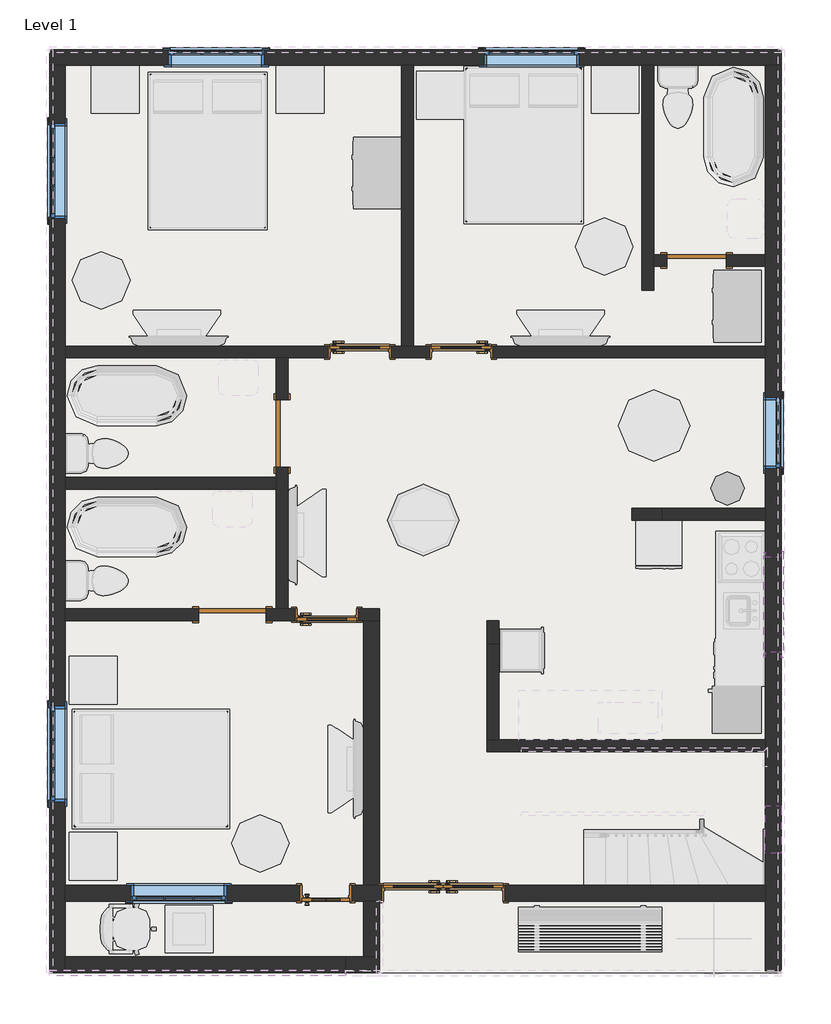
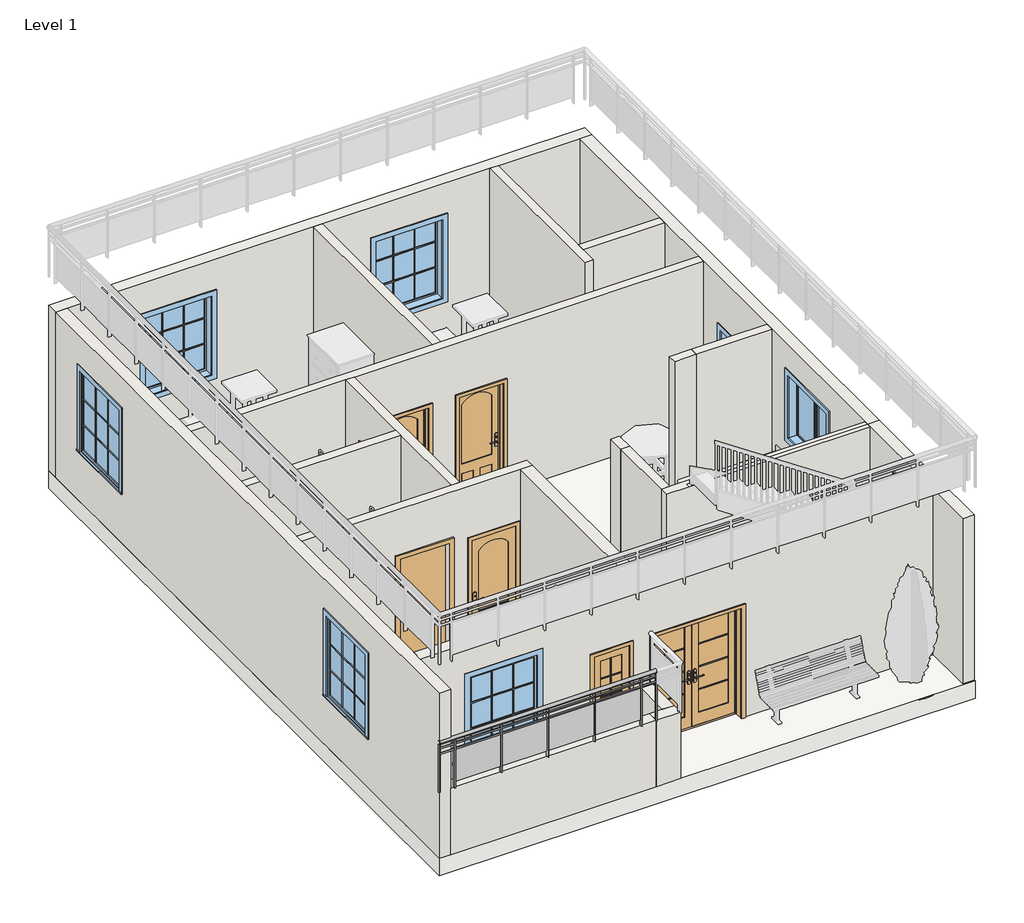
# One storey, part 1 of 4: 20 walls, 8 doors, 8 windows, 1 railing, 1 slab.
"""IFC4 building model written with IfcOpenShell, lengths in millimetres."""

from ifc_helpers import new_model, si_unit, point, frame, origin, origin_with_axes, place, context, project, spatial, polyline, ellipse_curve, trimmed, outline, extrude, faceted_brep, transform, mapped, element, save
from ifc_brep_helpers import plane_surface, extruded_surface, advanced_brep
from components import door_14b9be53, door_4b146b56, door_b03bd389, door_4bd6b2e0, door_255cab33, door_99d96fc5, door_b6e9fca3, window_29c06734, window_99fc0ff6, window_0862ab64, window_6846e476

model = new_model("IFC4")

# Units and contexts
model_context = context("Model", 3, world=origin())
ifc_project = project(units=[si_unit("LENGTHUNIT", "METRE", prefix="MILLI")], contexts=[model_context])

# Site, building, storey
site = spatial("IfcSite", under=ifc_project)
building = spatial("IfcBuilding", under=site)
storey = spatial("IfcBuildingStorey", under=building, Name="Level 1", Elevation=0.0)

# Doors
placement = place(None, origin())
door_shape = door_14b9be53(model_context)
element("IfcDoor", 1, ObjectType="30\" x 80\"", at=placement, inside=storey, context=model_context, shape_type="MappedRepresentation", body=[
    mapped(door_shape, transform((1456.0355823, 6247.8590324, 0.0), x_axis=(1.0, 0.0, 0.0), y_axis=(0.0, 1.0, 0.0), z_axis=(0.0, 0.0, 1.0))),
])
element("IfcDoor", 2, ObjectType="30\" x 80\"", at=placement, inside=storey, context=model_context, shape_type="MappedRepresentation", body=[
    mapped(door_shape, transform((-258.4644177, 2888.7090324, 0.0), x_axis=(-1.0, 0.0, 0.0), y_axis=(0.0, -1.0, 0.0), z_axis=(0.0, 0.0, 1.0))),
])
door_2_shape = door_4b146b56(model_context)
element("IfcDoor", 3, ObjectType="30\" x 80\"", at=placement, inside=storey, context=model_context, shape_type="MappedRepresentation", body=[
    mapped(door_2_shape, transform((160.6355823, 6247.8590324, 0.0), x_axis=(-1.0, 0.0, 0.0), y_axis=(0.0, -1.0, 0.0), z_axis=(0.0, 0.0, 1.0))),
])
door_3_shape = door_b03bd389(model_context)
element("IfcDoor", 4, ObjectType="Door-Exterior-Double-Full Glass-Wood_Clad : 60\" x 80\"", at=placement, inside=storey, context=model_context, shape_type="MappedRepresentation", body=[
    mapped(door_3_shape, transform((1227.4355823, -660.9409676, 0.0), x_axis=(1.0, 0.0, 0.0), y_axis=(0.0, 1.0, 0.0), z_axis=(0.0, 0.0, 1.0))),
])
door_4_shape = door_4bd6b2e0(model_context)
element("IfcDoor", 5, ObjectType="Door-Interior-Single-Full Glass-Wood : 24\" x 80\"", at=placement, inside=storey, context=model_context, shape_type="MappedRepresentation", body=[
    mapped(door_4_shape, transform((-271.1644177, -667.2909676, 0.0), x_axis=(1.0, 0.0, 0.0), y_axis=(0.0, 1.0, 0.0), z_axis=(0.0, 0.0, 1.0))),
])
door_5_shape = door_255cab33(model_context)
element("IfcDoor", 6, ObjectType="Single-Flush : 30\" x 80\"", at=placement, inside=storey, context=model_context, shape_type="MappedRepresentation", body=[
    mapped(door_5_shape, transform((4465.9355823, 7413.0840324, 0.0), x_axis=(-1.0, 0.0, 0.0), y_axis=(0.0, -1.0, 0.0), z_axis=(0.0, 0.0, 1.0))),
])
door_6_shape = door_99d96fc5(model_context)
element("IfcDoor", 7, ObjectType="Single-Flush : 34\" x 84\"", at=placement, inside=storey, context=model_context, shape_type="MappedRepresentation", body=[
    mapped(door_6_shape, transform((-829.9644177, 5203.2840324, 0.0), x_axis=(0.0, -1.0, 0.0), y_axis=(1.0, 0.0, 0.0), z_axis=(0.0, 0.0, 1.0))),
])
door_7_shape = door_b6e9fca3(model_context)
element("IfcDoor", 8, ObjectType="Single-Flush : 34\" x 84\"", at=placement, inside=storey, context=model_context, shape_type="MappedRepresentation", body=[
    mapped(door_7_shape, transform((-1464.9644177, 2891.8840324, 0.0), x_axis=(1.0, 0.0, 0.0), y_axis=(0.0, 1.0, 0.0), z_axis=(0.0, 0.0, 1.0))),
])

# Railing
element("IfcRailing", 9, ObjectType="Glass Panel - Bottom Fill", at=placement, inside=storey, context=model_context, shape_type="SolidModel", body=[
    advanced_brep(
    [(-3801.7644177, -1642.0159676, 2133.6), (-3801.7644177, -1718.2159676, 2133.6), (-17.1644177, -1642.0159676, 2133.6), (-17.1644177, -1718.2159676, 2133.6)],
    [
        (0, 1, ellipse_curve(frame((-3801.7644177, -1680.1159676, 2133.6), z_axis=(-1.0, 0.0, 0.0), x_axis=(0.0, -1.0, 0.0)), 38.1, 28.575)),
        (1, 0, ellipse_curve(frame((-3801.7644177, -1680.1159676, 2133.6), z_axis=(-1.0, 0.0, 0.0), x_axis=(0.0, -1.0, 0.0)), 38.1, 28.575)),
        (2, 3, ellipse_curve(frame((-17.1644177, -1680.1159676, 2133.6), z_axis=(1.0, 0.0, 0.0), x_axis=(0.0, -1.0, 0.0)), 38.1, 28.575)),
        (3, 2, ellipse_curve(frame((-17.1644177, -1680.1159676, 2133.6), z_axis=(1.0, 0.0, 0.0), x_axis=(0.0, -1.0, 0.0)), 38.1, 28.575)),
        (0, 2),
        (3, 1),
    ],
    [
        plane_surface(frame((-3801.7644177, -1680.1159676, 2133.6), z_axis=(-1.0, 0.0, 0.0), x_axis=(0.0, 1.0, 0.0))),
        plane_surface(frame((-17.1644177, -1680.1159676, 2133.6), z_axis=(1.0, 0.0, 0.0), x_axis=(0.0, 1.0, 0.0))),
        extruded_surface(trimmed(ellipse_curve(frame((-17.1644177, -1680.1159676, 2133.6), z_axis=(-1.0, 0.0, 0.0), x_axis=(0.0, -1.0, 0.0)), 38.1, 28.575), [point((-17.1644177, -1642.0159676, 2133.6))], [point((-17.1644177, -1718.2159676, 2133.6))], True, "CARTESIAN"), (-3784.6000000000004, 0.0, 0.0), 3784.6000000000004),
        extruded_surface(trimmed(ellipse_curve(frame((-17.1644177, -1680.1159676, 2133.6), z_axis=(-1.0, 0.0, 0.0), x_axis=(0.0, -1.0, 0.0)), 38.1, 28.575), [point((-17.1644177, -1718.2159676, 2133.6))], [point((-17.1644177, -1642.0159676, 2133.6))], True, "CARTESIAN"), (-3784.6000000000004, 0.0, 0.0), 3784.6000000000004),
    ],
    [
        (0, [[1, 2]]),
        (1, [[3, 4]]),
        (2, [[-1, 5, -4, 6]]),
        (3, [[-2, -6, -3, -5]]),
    ],
),
    extrude(outline(polyline([(-3801.7644177, -1692.8159676), (-3801.7644177, -1667.4159676), (-17.1644177, -1667.4159676), (-17.1644177, -1692.8159676), (-3801.7644177, -1692.8159676)])), frame((0.0, 0.0, 2019.3), z_axis=(0.0, 0.0, 1.0), x_axis=(1.0, 0.0, 0.0)), (0.0, 0.0, 1.0), 25.4),
    extrude(outline(polyline([(-3801.7644177, -1692.8159676), (-3801.7644177, -1667.4159676), (-17.1644177, -1667.4159676), (-17.1644177, -1692.8159676), (-3801.7644177, -1692.8159676)])), frame((0.0, 0.0, 1917.7), z_axis=(0.0, 0.0, 1.0), x_axis=(1.0, 0.0, 0.0)), (0.0, 0.0, 1.0), 25.4),
    extrude(outline(polyline([(-290.2144177, -1705.5159676), (-290.2144177, -1654.7159676), (-277.5144177, -1654.7159676), (-277.5144177, -1705.5159676), (-290.2144177, -1705.5159676)])), frame((0.0, 0.0, 1219.2), z_axis=(0.0, 0.0, 1.0), x_axis=(1.0, 0.0, 0.0)), (0.0, 0.0, 1.0), 885.6788223),
    extrude(outline(polyline([(-1096.6644177, -1673.5808106), (-283.8644177, -1673.5808106), (-283.8644177, -1679.9308106), (-1096.6644177, -1679.9308106), (-1096.6644177, -1673.5808106)])), frame((0.0, 0.0, 1320.8), z_axis=(0.0, 0.0, 1.0), x_axis=(1.0, 0.0, 0.0)), (0.0, 0.0, 1.0), 596.9),
    extrude(outline(polyline([(-1103.0144177, -1705.5159676), (-1103.0144177, -1654.7159676), (-1090.3144177, -1654.7159676), (-1090.3144177, -1705.5159676), (-1103.0144177, -1705.5159676)])), frame((0.0, 0.0, 1219.2), z_axis=(0.0, 0.0, 1.0), x_axis=(1.0, 0.0, 0.0)), (0.0, 0.0, 1.0), 885.6788223),
    extrude(outline(polyline([(-1909.4644177, -1673.5808106), (-1096.6644177, -1673.5808106), (-1096.6644177, -1679.9308106), (-1909.4644177, -1679.9308106), (-1909.4644177, -1673.5808106)])), frame((0.0, 0.0, 1320.8), z_axis=(0.0, 0.0, 1.0), x_axis=(1.0, 0.0, 0.0)), (0.0, 0.0, 1.0), 596.9),
    extrude(outline(polyline([(-1915.8144177, -1705.5159676), (-1915.8144177, -1654.7159676), (-1903.1144177, -1654.7159676), (-1903.1144177, -1705.5159676), (-1915.8144177, -1705.5159676)])), frame((0.0, 0.0, 1219.2), z_axis=(0.0, 0.0, 1.0), x_axis=(1.0, 0.0, 0.0)), (0.0, 0.0, 1.0), 885.6788223),
    extrude(outline(polyline([(-2722.2644177, -1673.5808106), (-1909.4644177, -1673.5808106), (-1909.4644177, -1679.9308106), (-2722.2644177, -1679.9308106), (-2722.2644177, -1673.5808106)])), frame((0.0, 0.0, 1320.8), z_axis=(0.0, 0.0, 1.0), x_axis=(1.0, 0.0, 0.0)), (0.0, 0.0, 1.0), 596.9),
    extrude(outline(polyline([(-2728.6144177, -1705.5159676), (-2728.6144177, -1654.7159676), (-2715.9144177, -1654.7159676), (-2715.9144177, -1705.5159676), (-2728.6144177, -1705.5159676)])), frame((0.0, 0.0, 1219.2), z_axis=(0.0, 0.0, 1.0), x_axis=(1.0, 0.0, 0.0)), (0.0, 0.0, 1.0), 885.6788223),
    extrude(outline(polyline([(-3535.0644177, -1673.5808106), (-2722.2644177, -1673.5808106), (-2722.2644177, -1679.9308106), (-3535.0644177, -1679.9308106), (-3535.0644177, -1673.5808106)])), frame((0.0, 0.0, 1320.8), z_axis=(0.0, 0.0, 1.0), x_axis=(1.0, 0.0, 0.0)), (0.0, 0.0, 1.0), 596.9),
    extrude(outline(polyline([(-3541.4144177, -1705.5159676), (-3541.4144177, -1654.7159676), (-3528.7144177, -1654.7159676), (-3528.7144177, -1705.5159676), (-3541.4144177, -1705.5159676)])), frame((0.0, 0.0, 1219.2), z_axis=(0.0, 0.0, 1.0), x_axis=(1.0, 0.0, 0.0)), (0.0, 0.0, 1.0), 885.6788223),
    extrude(outline(polyline([(-29.8644177, -1689.6409676), (-29.8644177, -1670.5909676), (-10.8144177, -1670.5909676), (-10.8144177, -1689.6409676), (-29.8644177, -1689.6409676)])), frame((0.0, 0.0, 1219.2), z_axis=(0.0, 0.0, 1.0), x_axis=(1.0, 0.0, 0.0)), (0.0, 0.0, 1.0), 885.6788223),
    extrude(outline(polyline([(-3808.1144177, -1689.6409676), (-3808.1144177, -1670.5909676), (-3789.0644177, -1670.5909676), (-3789.0644177, -1689.6409676), (-3808.1144177, -1689.6409676)])), frame((0.0, 0.0, 1219.2), z_axis=(0.0, 0.0, 1.0), x_axis=(1.0, 0.0, 0.0)), (0.0, 0.0, 1.0), 885.6788223),
])

# Slab
element("IfcSlab", 10, at=placement, inside=storey, context=model_context, shape_type="SweptSolid", body=[
    extrude(outline(polyline([(-3801.7644177, -1680.1159676), (-3801.7644177, 10105.4840324), (5545.4355823, 10105.4840324), (5545.4355823, -1680.1159676), (-3801.7644177, -1680.1159676)])), frame((0.0, 0.0, -323.85), z_axis=(0.0, 0.0, 1.0), x_axis=(1.0, 0.0, 0.0)), (0.0, 0.0, 1.0), 323.85),
])

# Walls
element("IfcWall", 11, ObjectType="Generic - 8\"", at=placement, inside=storey, context=model_context, shape_type="Brep", body=[
    faceted_brep([(-3801.7644177, 9902.2840324, 0.0), (-3598.5644177, 9902.2840324, 0.0), (694.0355823, 9902.2840324, 0.0), (846.4355823, 9902.2840324, 0.0), (3767.4355823, 9902.2840324, 0.0), (3919.8355823, 9902.2840324, 0.0), (5342.2355823, 9902.2840324, 0.0), (5545.4355823, 9902.2840324, 0.0), (5545.4355823, 9902.2840324, 3048.0), (5342.2355823, 9902.2840324, 3048.0), (3919.8355823, 9902.2840324, 3048.0), (3767.4355823, 9902.2840324, 3048.0), (846.4355823, 9902.2840324, 3048.0), (694.0355823, 9902.2840324, 3048.0), (-3598.5644177, 9902.2840324, 3048.0), (-3801.7644177, 9902.2840324, 3048.0), (-1058.5644177, 9902.2840324, 2438.4), (-1058.5644177, 9902.2840324, 914.4), (-2277.7644177, 9902.2840324, 914.4), (-2277.7644177, 9902.2840324, 2438.4), (2967.3355823, 9902.2840324, 2438.4), (2967.3355823, 9902.2840324, 914.4), (1748.1355823, 9902.2840324, 914.4), (1748.1355823, 9902.2840324, 2438.4), (-3801.7644177, 10105.4840324, 0.0), (-3801.7644177, 10105.4840324, 3048.0), (5545.4355823, 10105.4840324, 3048.0), (5545.4355823, 10105.4840324, 0.0), (-1058.5644177, 10105.4840324, 2438.4), (-2277.7644177, 10105.4840324, 2438.4), (-2277.7644177, 10105.4840324, 914.4), (-1058.5644177, 10105.4840324, 914.4), (2967.3355823, 10105.4840324, 2438.4), (1748.1355823, 10105.4840324, 2438.4), (1748.1355823, 10105.4840324, 914.4), (2967.3355823, 10105.4840324, 914.4)], [[[0, 1, 2, 3, 4, 5, 6, 7, 8, 9, 10, 11, 12, 13, 14, 15], [16, 17, 18, 19], [20, 21, 22, 23]], [[24, 25, 26, 27], [28, 29, 30, 31], [32, 33, 34, 35]], [[7, 6, 5, 4, 3, 2, 1, 0, 24, 27]], [[0, 15, 25, 24]], [[8, 7, 27, 26]], [[15, 14, 13, 12, 11, 10, 9, 8, 26, 25]], [[17, 16, 28, 31]], [[18, 17, 31, 30]], [[19, 18, 30, 29]], [[16, 19, 29, 28]], [[21, 20, 32, 35]], [[22, 21, 35, 34]], [[23, 22, 34, 33]], [[20, 23, 33, 32]]]),
])
element("IfcWall", 12, ObjectType="Generic - 8\"", at=placement, inside=storey, context=model_context, shape_type="Brep", body=[
    faceted_brep([(-3801.7644177, 9902.2840324, 0.0), (-3801.7644177, -1680.1159676, 0.0), (-3801.7644177, -1680.1159676, 3048.0), (-3801.7644177, 9902.2840324, 3048.0), (-3801.7644177, 1723.4840324, 2438.4), (-3801.7644177, 504.2840324, 2438.4), (-3801.7644177, 504.2840324, 914.4), (-3801.7644177, 1723.4840324, 914.4), (-3801.7644177, 9165.6840324, 2438.4), (-3801.7644177, 7946.4840324, 2438.4), (-3801.7644177, 7946.4840324, 914.4), (-3801.7644177, 9165.6840324, 914.4), (-3598.5644177, 9902.2840324, 0.0), (-3598.5644177, 9902.2840324, 3048.0), (-3598.5644177, 6320.8840324, 3048.0), (-3598.5644177, 6168.4840324, 3048.0), (-3598.5644177, 4644.4840324, 3048.0), (-3598.5644177, 4492.0840324, 3048.0), (-3598.5644177, 2968.0840324, 3048.0), (-3598.5644177, 2815.6840324, 3048.0), (-3598.5644177, -562.5159676, 3048.0), (-3598.5644177, -765.7159676, 3048.0), (-3598.5644177, -1680.1159676, 3048.0), (-3598.5644177, -1680.1159676, 1219.2), (-3598.5644177, -1680.1159676, 0.0), (-3598.5644177, -1476.9159676, 0.0), (-3598.5644177, -765.7159676, 0.0), (-3598.5644177, -562.5159676, 0.0), (-3598.5644177, 2815.6840324, 0.0), (-3598.5644177, 2968.0840324, 0.0), (-3598.5644177, 4492.0840324, 0.0), (-3598.5644177, 4644.4840324, 0.0), (-3598.5644177, 6168.4840324, 0.0), (-3598.5644177, 6320.8840324, 0.0), (-3598.5644177, 1723.4840324, 2438.4), (-3598.5644177, 1723.4840324, 914.4), (-3598.5644177, 504.2840324, 914.4), (-3598.5644177, 504.2840324, 2438.4), (-3598.5644177, 9165.6840324, 2438.4), (-3598.5644177, 9165.6840324, 914.4), (-3598.5644177, 7946.4840324, 914.4), (-3598.5644177, 7946.4840324, 2438.4)], [[[0, 1, 2, 3], [4, 5, 6, 7], [8, 9, 10, 11]], [[12, 13, 14, 15, 16, 17, 18, 19, 20, 21, 22, 23, 24, 25, 26, 27, 28, 29, 30, 31, 32, 33], [34, 35, 36, 37], [38, 39, 40, 41]], [[1, 0, 12, 33, 32, 31, 30, 29, 28, 27, 26, 25, 24]], [[0, 3, 13, 12]], [[2, 1, 24, 23, 22]], [[3, 2, 22, 21, 20, 19, 18, 17, 16, 15, 14, 13]], [[35, 34, 4, 7]], [[36, 35, 7, 6]], [[37, 36, 6, 5]], [[34, 37, 5, 4]], [[39, 38, 8, 11]], [[40, 39, 11, 10]], [[41, 40, 10, 9]], [[38, 41, 9, 8]]]),
])
element("IfcWall", 13, ObjectType="Generic - 8\"", at=placement, inside=storey, context=model_context, shape_type="Brep", body=[
    faceted_brep([(5545.4355823, -1654.7159676, 0.0), (5545.4355823, 9902.2840324, 0.0), (5545.4355823, 9902.2840324, 3048.0), (5545.4355823, 1215.4840324, 3048.0), (5545.4355823, -537.1159676, 3048.0), (5545.4355823, -1654.7159676, 3048.0), (5545.4355823, 4752.4340324, 2133.6), (5545.4355823, 5666.8340324, 2133.6), (5545.4355823, 5666.8340324, 914.4), (5545.4355823, 4752.4340324, 914.4), (5545.4355823, 2409.2840324, 2540.0), (5545.4355823, 3628.4840324, 2540.0), (5545.4355823, 3628.4840324, 1320.8), (5545.4355823, 2409.2840324, 1320.8), (5545.4355823, -156.1159676, 2667.0), (5545.4355823, 453.4840324, 2667.0), (5545.4355823, 453.4840324, 2057.4), (5545.4355823, -156.1159676, 2057.4), (5342.2355823, -1654.7159676, 0.0), (5342.2355823, -1654.7159676, 3048.0), (5342.2355823, -765.7159676, 3048.0), (5342.2355823, -562.5159676, 3048.0), (5342.2355823, -537.1159676, 3048.0), (5342.2355823, 1139.2840324, 3048.0), (5342.2355823, 1215.4840324, 3048.0), (5342.2355823, 1291.6840324, 3048.0), (5342.2355823, 4098.3840324, 3048.0), (5342.2355823, 4250.7840324, 3048.0), (5342.2355823, 6168.4840324, 3048.0), (5342.2355823, 6320.8840324, 3048.0), (5342.2355823, 7336.8840324, 3048.0), (5342.2355823, 7489.2840324, 3048.0), (5342.2355823, 9902.2840324, 3048.0), (5342.2355823, 9902.2840324, 0.0), (5342.2355823, 7489.2840324, 0.0), (5342.2355823, 7336.8840324, 0.0), (5342.2355823, 6320.8840324, 0.0), (5342.2355823, 6168.4840324, 0.0), (5342.2355823, 4250.7840324, 0.0), (5342.2355823, 4098.3840324, 0.0), (5342.2355823, 1291.6840324, 0.0), (5342.2355823, 1139.2840324, 0.0), (5342.2355823, -562.5159676, 0.0), (5342.2355823, -765.7159676, 0.0), (5342.2355823, 4752.4340324, 2133.6), (5342.2355823, 4752.4340324, 914.4), (5342.2355823, 5666.8340324, 914.4), (5342.2355823, 5666.8340324, 2133.6), (5342.2355823, 2409.2840324, 2540.0), (5342.2355823, 2409.2840324, 1320.8), (5342.2355823, 3628.4840324, 1320.8), (5342.2355823, 3628.4840324, 2540.0), (5342.2355823, -156.1159676, 2667.0), (5342.2355823, -156.1159676, 2057.4), (5342.2355823, 453.4840324, 2057.4), (5342.2355823, 453.4840324, 2667.0)], [[[0, 1, 2, 3, 4, 5], [6, 7, 8, 9], [10, 11, 12, 13], [14, 15, 16, 17]], [[18, 19, 20, 21, 22, 23, 24, 25, 26, 27, 28, 29, 30, 31, 32, 33, 34, 35, 36, 37, 38, 39, 40, 41, 42, 43], [44, 45, 46, 47], [48, 49, 50, 51], [52, 53, 54, 55]], [[1, 0, 18, 43, 42, 41, 40, 39, 38, 37, 36, 35, 34, 33]], [[0, 5, 19, 18]], [[4, 3, 24, 23, 22]], [[2, 1, 33, 32]], [[5, 4, 22, 21, 20, 19]], [[3, 2, 32, 31, 30, 29, 28, 27, 26, 25, 24]], [[45, 44, 6, 9]], [[46, 45, 9, 8]], [[47, 46, 8, 7]], [[44, 47, 7, 6]], [[49, 48, 10, 13]], [[50, 49, 13, 12]], [[51, 50, 12, 11]], [[48, 51, 11, 10]], [[53, 52, 14, 17]], [[54, 53, 17, 16]], [[55, 54, 16, 15]], [[52, 55, 15, 14]]]),
])
element("IfcWall", 14, ObjectType="Generic - 8\"", at=placement, inside=storey, context=model_context, shape_type="Brep", body=[
    faceted_brep([(-3598.5644177, -562.5159676, 0.0), (-3598.5644177, -562.5159676, 3048.0), (211.4355823, -562.5159676, 3048.0), (414.6355823, -562.5159676, 3048.0), (5342.2355823, -562.5159676, 3048.0), (5342.2355823, -562.5159676, 0.0), (2014.8355823, -562.5159676, 0.0), (2014.8355823, -562.5159676, 2057.4), (440.0355823, -562.5159676, 2057.4), (440.0355823, -562.5159676, 0.0), (414.6355823, -562.5159676, 0.0), (211.4355823, -562.5159676, 0.0), (59.0355823, -562.5159676, 0.0), (59.0355823, -562.5159676, 2057.4), (-601.3644177, -562.5159676, 2057.4), (-601.3644177, -562.5159676, 0.0), (-2760.3644177, -562.5159676, 2438.4), (-2760.3644177, -562.5159676, 914.4), (-1541.1644177, -562.5159676, 914.4), (-1541.1644177, -562.5159676, 2438.4), (-3598.5644177, -765.7159676, 3048.0), (-3598.5644177, -765.7159676, 0.0), (-601.3644177, -765.7159676, 0.0), (-601.3644177, -765.7159676, 2057.4), (59.0355823, -765.7159676, 2057.4), (59.0355823, -765.7159676, 0.0), (211.4355823, -765.7159676, 0.0), (414.6355823, -765.7159676, 0.0), (440.0355823, -765.7159676, 0.0), (440.0355823, -765.7159676, 2057.4), (2014.8355823, -765.7159676, 2057.4), (2014.8355823, -765.7159676, 0.0), (5342.2355823, -765.7159676, 0.0), (5342.2355823, -765.7159676, 3048.0), (-2760.3644177, -765.7159676, 2438.4), (-1541.1644177, -765.7159676, 2438.4), (-1541.1644177, -765.7159676, 914.4), (-2760.3644177, -765.7159676, 914.4)], [[[0, 1, 2, 3, 4, 5, 6, 7, 8, 9, 10, 11, 12, 13, 14, 15], [16, 17, 18, 19]], [[20, 21, 22, 23, 24, 25, 26, 27, 28, 29, 30, 31, 32, 33], [34, 35, 36, 37]], [[5, 32, 31, 6]], [[21, 0, 15, 22]], [[9, 28, 27, 26, 25, 12, 11, 10]], [[1, 0, 21, 20]], [[5, 4, 33, 32]], [[30, 7, 6, 31]], [[7, 30, 29, 8]], [[8, 29, 28, 9]], [[4, 3, 2, 1, 20, 33]], [[24, 13, 12, 25]], [[13, 24, 23, 14]], [[14, 23, 22, 15]], [[17, 16, 34, 37]], [[18, 17, 37, 36]], [[19, 18, 36, 35]], [[16, 19, 35, 34]]]),
])
element("IfcWall", 15, ObjectType="Generic - 8\"", at=placement, inside=storey, context=model_context, shape_type="SweptSolid", body=[
    extrude(outline(polyline([(414.6355823, 2815.6840324), (414.6355823, -562.5159676), (211.4355823, -562.5159676), (211.4355823, 2815.6840324), (414.6355823, 2815.6840324)])), origin_with_axes(), (0.0, 0.0, 1.0), 3048.0),
])
element("IfcWall", 16, ObjectType="Generic - 8\"", at=placement, inside=storey, context=model_context, shape_type="SweptSolid", body=[
    extrude(outline(polyline([(-17.1644177, -1680.1159676), (-3598.5644177, -1680.1159676), (-3598.5644177, -1476.9159676), (-17.1644177, -1476.9159676), (-17.1644177, -1680.1159676)])), origin_with_axes(), (0.0, 0.0, 1.0), 1219.2),
])
element("IfcWall", 17, ObjectType="Generic - 8\"", at=placement, inside=storey, context=model_context, shape_type="Brep", body=[
    faceted_brep([(-17.1644177, -1680.1159676, 0.0), (414.6355823, -1680.1159676, 0.0), (414.6355823, -1680.1159676, 1219.2), (-17.1644177, -1680.1159676, 1219.2), (-17.1644177, -1476.9159676, 0.0), (-17.1644177, -1476.9159676, 1219.2), (211.4355823, -1476.9159676, 1219.2), (414.6355823, -1476.9159676, 1219.2), (414.6355823, -1476.9159676, 0.0), (211.4355823, -1476.9159676, 0.0)], [[[0, 1, 2, 3]], [[4, 5, 6, 7, 8, 9]], [[1, 0, 4, 9, 8]], [[3, 2, 7, 6, 5]], [[0, 3, 5, 4]], [[2, 1, 8, 7]]]),
])
element("IfcWall", 18, ObjectType="Generic - 8\"", at=placement, inside=storey, context=model_context, shape_type="SweptSolid", body=[
    extrude(outline(polyline([(414.6355823, -765.7159676), (414.6355823, -1476.9159676), (211.4355823, -1476.9159676), (211.4355823, -765.7159676), (414.6355823, -765.7159676)])), origin_with_axes(), (0.0, 0.0, 1.0), 1219.2),
])
element("IfcWall", 19, ObjectType="INNER WALL", at=placement, inside=storey, context=model_context, shape_type="Brep", body=[
    faceted_brep([(-3598.5644177, 6320.8840324, 0.0), (-3598.5644177, 6320.8840324, 3048.0), (694.0355823, 6320.8840324, 3048.0), (846.4355823, 6320.8840324, 3048.0), (5342.2355823, 6320.8840324, 3048.0), (5342.2355823, 6320.8840324, 0.0), (1862.4355823, 6320.8840324, 0.0), (1862.4355823, 6320.8840324, 2057.4), (1049.6355823, 6320.8840324, 2057.4), (1049.6355823, 6320.8840324, 0.0), (846.4355823, 6320.8840324, 0.0), (694.0355823, 6320.8840324, 0.0), (567.0355823, 6320.8840324, 0.0), (567.0355823, 6320.8840324, 2057.4), (-245.7644177, 6320.8840324, 2057.4), (-245.7644177, 6320.8840324, 0.0), (-3598.5644177, 6168.4840324, 3048.0), (-3598.5644177, 6168.4840324, 0.0), (-906.1644177, 6168.4840324, 0.0), (-753.7644177, 6168.4840324, 0.0), (-245.7644177, 6168.4840324, 0.0), (-245.7644177, 6168.4840324, 2057.4), (567.0355823, 6168.4840324, 2057.4), (567.0355823, 6168.4840324, 0.0), (1049.6355823, 6168.4840324, 0.0), (1049.6355823, 6168.4840324, 2057.4), (1862.4355823, 6168.4840324, 2057.4), (1862.4355823, 6168.4840324, 0.0), (5342.2355823, 6168.4840324, 0.0), (5342.2355823, 6168.4840324, 3048.0), (-753.7644177, 6168.4840324, 3048.0), (-906.1644177, 6168.4840324, 3048.0)], [[[0, 1, 2, 3, 4, 5, 6, 7, 8, 9, 10, 11, 12, 13, 14, 15]], [[16, 17, 18, 19, 20, 21, 22, 23, 24, 25, 26, 27, 28, 29, 30, 31]], [[5, 28, 27, 6]], [[17, 0, 15, 20, 19, 18]], [[9, 24, 23, 12, 11, 10]], [[1, 0, 17, 16]], [[5, 4, 29, 28]], [[26, 7, 6, 27]], [[7, 26, 25, 8]], [[8, 25, 24, 9]], [[14, 21, 20, 15]], [[21, 14, 13, 22]], [[22, 13, 12, 23]], [[4, 3, 2, 1, 16, 31, 30, 29]]]),
])
element("IfcWall", 20, ObjectType="INNER WALL", at=placement, inside=storey, context=model_context, shape_type="SweptSolid", body=[
    extrude(outline(polyline([(694.0355823, 6320.8840324), (694.0355823, 9902.2840324), (846.4355823, 9902.2840324), (846.4355823, 6320.8840324), (694.0355823, 6320.8840324)])), origin_with_axes(), (0.0, 0.0, 1.0), 3048.0),
])
element("IfcWall", 21, ObjectType="INNER WALL", at=placement, inside=storey, context=model_context, shape_type="Brep", body=[
    faceted_brep([(-906.1644177, 4771.4840324, 2133.6), (-906.1644177, 4771.4840324, 0.0), (-906.1644177, 4644.4840324, 0.0), (-906.1644177, 4492.0840324, 0.0), (-906.1644177, 2968.0840324, 0.0), (-906.1644177, 2968.0840324, 3048.0), (-906.1644177, 4492.0840324, 3048.0), (-906.1644177, 4644.4840324, 3048.0), (-906.1644177, 6168.4840324, 3048.0), (-906.1644177, 6168.4840324, 0.0), (-906.1644177, 5635.0840324, 0.0), (-906.1644177, 5635.0840324, 2133.6), (-753.7644177, 2968.0840324, 0.0), (-753.7644177, 4771.4840324, 0.0), (-753.7644177, 4771.4840324, 2133.6), (-753.7644177, 5635.0840324, 2133.6), (-753.7644177, 5635.0840324, 0.0), (-753.7644177, 6168.4840324, 0.0), (-753.7644177, 6168.4840324, 3048.0), (-753.7644177, 2968.0840324, 3048.0)], [[[0, 1, 2, 3, 4, 5, 6, 7, 8, 9, 10, 11]], [[12, 13, 14, 15, 16, 17, 18, 19]], [[10, 9, 17, 16]], [[4, 3, 2, 1, 13, 12]], [[9, 8, 18, 17]], [[5, 4, 12, 19]], [[14, 13, 1, 0]], [[15, 14, 0, 11]], [[16, 15, 11, 10]], [[8, 7, 6, 5, 19, 18]]]),
])
element("IfcWall", 22, ObjectType="INNER WALL", at=placement, inside=storey, context=model_context, shape_type="SweptSolid", body=[
    extrude(outline(polyline([(-3598.5644177, 4644.4840324), (-906.1644177, 4644.4840324), (-906.1644177, 4492.0840324), (-3598.5644177, 4492.0840324), (-3598.5644177, 4644.4840324)])), origin_with_axes(), (0.0, 0.0, 1.0), 3048.0),
])
element("IfcWall", 23, ObjectType="INNER WALL", at=placement, inside=storey, context=model_context, shape_type="Brep", body=[
    faceted_brep([(5342.2355823, 1291.6840324, 0.0), (1938.6355823, 1291.6840324, 0.0), (1786.2355823, 1291.6840324, 0.0), (1786.2355823, 1291.6840324, 3048.0), (1938.6355823, 1291.6840324, 3048.0), (5342.2355823, 1291.6840324, 3048.0), (5342.2355823, 1139.2840324, 0.0), (5342.2355823, 1139.2840324, 3048.0), (2192.6355823, 1139.2840324, 3048.0), (1786.2355823, 1139.2840324, 3048.0), (1786.2355823, 1139.2840324, 0.0), (5342.2355823, 1215.4840324, 3048.0), (1786.2355823, 1215.4840324, 3048.0), (2192.6355823, 1215.4840324, 3048.0)], [[[0, 1, 2, 3, 4, 5]], [[6, 7, 8, 9, 10]], [[2, 1, 0, 6, 10]], [[0, 5, 11, 7, 6]], [[3, 2, 10, 9, 12]], [[8, 7, 11, 13]], [[3, 12, 9, 8, 13, 11, 5, 4]]]),
])
element("IfcWall", 24, ObjectType="INNER WALL", at=placement, inside=storey, context=model_context, shape_type="SweptSolid", body=[
    extrude(outline(polyline([(1938.6355823, 2510.8840324), (1938.6355823, 1291.6840324), (1786.2355823, 1291.6840324), (1786.2355823, 2510.8840324), (1938.6355823, 2510.8840324)])), origin_with_axes(), (0.0, 0.0, 1.0), 3048.0),
])
element("IfcWall", 25, ObjectType="INNER WALL", at=placement, inside=storey, context=model_context, shape_type="Brep", body=[
    faceted_brep([(-3598.5644177, 2968.0840324, 0.0), (-3598.5644177, 2968.0840324, 3048.0), (-906.1644177, 2968.0840324, 3048.0), (-753.7644177, 2968.0840324, 3048.0), (414.6355823, 2968.0840324, 3048.0), (414.6355823, 2968.0840324, 0.0), (147.9355823, 2968.0840324, 0.0), (147.9355823, 2968.0840324, 2057.4), (-664.8644177, 2968.0840324, 2057.4), (-664.8644177, 2968.0840324, 0.0), (-753.7644177, 2968.0840324, 0.0), (-906.1644177, 2968.0840324, 0.0), (-1033.1644177, 2968.0840324, 0.0), (-1033.1644177, 2968.0840324, 2133.6), (-1896.7644177, 2968.0840324, 2133.6), (-1896.7644177, 2968.0840324, 0.0), (-3598.5644177, 2815.6840324, 3048.0), (-3598.5644177, 2815.6840324, 0.0), (-1896.7644177, 2815.6840324, 0.0), (-1896.7644177, 2815.6840324, 2133.6), (-1033.1644177, 2815.6840324, 2133.6), (-1033.1644177, 2815.6840324, 0.0), (-664.8644177, 2815.6840324, 0.0), (-664.8644177, 2815.6840324, 2057.4), (147.9355823, 2815.6840324, 2057.4), (147.9355823, 2815.6840324, 0.0), (211.4355823, 2815.6840324, 0.0), (414.6355823, 2815.6840324, 0.0), (414.6355823, 2815.6840324, 3048.0), (211.4355823, 2815.6840324, 3048.0)], [[[0, 1, 2, 3, 4, 5, 6, 7, 8, 9, 10, 11, 12, 13, 14, 15]], [[16, 17, 18, 19, 20, 21, 22, 23, 24, 25, 26, 27, 28, 29]], [[17, 0, 15, 18]], [[5, 27, 26, 25, 6]], [[21, 12, 11, 10, 9, 22]], [[1, 0, 17, 16]], [[5, 4, 28, 27]], [[13, 12, 21, 20]], [[14, 13, 20, 19]], [[15, 14, 19, 18]], [[8, 23, 22, 9]], [[23, 8, 7, 24]], [[24, 7, 6, 25]], [[4, 3, 2, 1, 16, 29, 28]]]),
])
element("IfcWall", 26, ObjectType="INNER WALL", at=placement, inside=storey, context=model_context, shape_type="SweptSolid", body=[
    extrude(outline(polyline([(4021.4355823, 4250.7840324), (5342.2355823, 4250.7840324), (5342.2355823, 4098.3840324), (4021.4355823, 4098.3840324), (4021.4355823, 4250.7840324)])), origin_with_axes(), (0.0, 0.0, 1.0), 3048.0),
])
element("IfcWall", 27, ObjectType="INNER WALL", at=placement, inside=storey, context=model_context, shape_type="Brep", body=[
    faceted_brep([(3767.4355823, 9902.2840324, 0.0), (3767.4355823, 7032.0840324, 0.0), (3767.4355823, 7032.0840324, 3048.0), (3767.4355823, 9902.2840324, 3048.0), (3919.8355823, 9902.2840324, 0.0), (3919.8355823, 9902.2840324, 3048.0), (3919.8355823, 7489.2840324, 3048.0), (3919.8355823, 7336.8840324, 3048.0), (3919.8355823, 7032.0840324, 3048.0), (3919.8355823, 7032.0840324, 0.0), (3919.8355823, 7336.8840324, 0.0), (3919.8355823, 7489.2840324, 0.0)], [[[0, 1, 2, 3]], [[4, 5, 6, 7, 8, 9, 10, 11]], [[1, 0, 4, 11, 10, 9]], [[2, 1, 9, 8]], [[0, 3, 5, 4]], [[3, 2, 8, 7, 6, 5]]]),
])
element("IfcWall", 28, ObjectType="INNER WALL", at=placement, inside=storey, context=model_context, shape_type="SweptSolid", body=[
    extrude(outline(polyline([(0.0, 3919.8355823), (0.0, 4084.9355823), (2032.0, 4084.9355823), (2032.0, 4846.9355823), (0.0, 4846.9355823), (0.0, 5342.2355823), (3048.0, 5342.2355823), (3048.0, 3919.8355823), (0.0, 3919.8355823)])), frame((0.0, 7336.8840324, 0.0), z_axis=(0.0, 1.0, 0.0), x_axis=(0.0, 0.0, 1.0)), (0.0, 0.0, 1.0), 152.4),
])
element("IfcWall", 29, ObjectType="INNER WALL", at=placement, inside=storey, context=model_context, shape_type="SweptSolid", body=[
    extrude(outline(polyline([(3640.4355823, 4250.7840324), (4021.4355823, 4250.7840324), (4021.4355823, 4098.3840324), (3640.4355823, 4098.3840324), (3640.4355823, 4250.7840324)])), origin_with_axes(), (0.0, 0.0, 1.0), 3048.0),
])
element("IfcWall", 30, ObjectType="INNER WALL", at=placement, inside=storey, context=model_context, shape_type="SweptSolid", body=[
    extrude(outline(polyline([(1938.6355823, 2815.6840324), (1938.6355823, 2510.8840324), (1786.2355823, 2510.8840324), (1786.2355823, 2815.6840324), (1938.6355823, 2815.6840324)])), origin_with_axes(), (0.0, 0.0, 1.0), 3048.0),
])

# Windows
window_shape = window_29c06734(model_context)
element("IfcWindow", 31, ObjectType="Casement 3x3 with Trim : 36\" x 48\"", at=placement, inside=storey, context=model_context, shape_type="MappedRepresentation", body=[
    mapped(window_shape, transform((5443.8355823, 5209.6340324, 0.0), x_axis=(0.0, -1.0, 0.0), y_axis=(1.0, 0.0, 0.0), z_axis=(0.0, 0.0, 1.0))),
])
window_2_shape = window_99fc0ff6(model_context)
element("IfcWindow", 32, ObjectType="Casement 3x3 with Trim : 48\" x 60\"", at=placement, inside=storey, context=model_context, shape_type="MappedRepresentation", body=[
    mapped(window_2_shape, transform((-2150.7644177, -664.1159676, 609.6), x_axis=(-1.0, 0.0, 0.0), y_axis=(0.0, -1.0, 0.0), z_axis=(0.0, 0.0, 1.0))),
])
element("IfcWindow", 33, ObjectType="Casement 3x3 with Trim : 48\" x 60\"", at=placement, inside=storey, context=model_context, shape_type="MappedRepresentation", body=[
    mapped(window_2_shape, transform((-3700.1644177, 1113.8840324, 609.6), x_axis=(0.0, 1.0, 0.0), y_axis=(-1.0, 0.0, 0.0), z_axis=(0.0, 0.0, 1.0))),
])
element("IfcWindow", 34, ObjectType="Casement 3x3 with Trim : 48\" x 60\"", at=placement, inside=storey, context=model_context, shape_type="MappedRepresentation", body=[
    mapped(window_2_shape, transform((-3700.1644177, 8556.0840324, 609.6), x_axis=(0.0, 1.0, 0.0), y_axis=(-1.0, 0.0, 0.0), z_axis=(0.0, 0.0, 1.0))),
])
element("IfcWindow", 35, ObjectType="Casement 3x3 with Trim : 48\" x 60\"", at=placement, inside=storey, context=model_context, shape_type="MappedRepresentation", body=[
    mapped(window_2_shape, transform((-1668.1644177, 10003.8840324, 609.6), x_axis=(1.0, 0.0, 0.0), y_axis=(0.0, 1.0, 0.0), z_axis=(0.0, 0.0, 1.0))),
])
element("IfcWindow", 36, ObjectType="Casement 3x3 with Trim : 48\" x 60\"", at=placement, inside=storey, context=model_context, shape_type="MappedRepresentation", body=[
    mapped(window_2_shape, transform((2357.7355823, 10003.8840324, 609.6), x_axis=(1.0, 0.0, 0.0), y_axis=(0.0, 1.0, 0.0), z_axis=(0.0, 0.0, 1.0))),
])
window_3_shape = window_0862ab64(model_context)
element("IfcWindow", 37, ObjectType="Casement Dbl with Trim : 48\" x 48\"", at=placement, inside=storey, context=model_context, shape_type="MappedRepresentation", body=[
    mapped(window_3_shape, transform((5424.7855823, 3018.8840324, 406.4), x_axis=(0.0, -1.0, 0.0), y_axis=(1.0, 0.0, 0.0), z_axis=(0.0, 0.0, 1.0))),
])
window_4_shape = window_6846e476(model_context)
element("IfcWindow", 38, ObjectType="Fixed : 24\" x 24\"", at=placement, inside=storey, context=model_context, shape_type="MappedRepresentation", body=[
    mapped(window_4_shape, transform((5443.8355823, 110.5840324, 1143.0), x_axis=(0.0, -1.0, 0.0), y_axis=(1.0, 0.0, 0.0), z_axis=(0.0, 0.0, 1.0))),
])

save(model, "model.ifc")

# Revit data of these elements
# Type "30\" x 80\""
#   Type Mark = "9"
#   Assembly Code = "B2030100"
#   Analytic Construction = "French door, wood frame with single glass"
#   Threshold Offset [instance default] = 0' - 0 1/2"
#   Thickness = 0' - 1 3/8"
#   Thermal Resistance (R) = 1.0696 (h·ft²·°F)/BTU
#   Swing Angle [instance default] = 90.00°
#   Stiles = 0' - 4 3/4"
#   Rough Width = 2' - 8"
#   Rough Height = 6' - 9"
#   Radius = 1' - 1.00625"
#   Lock Rail = 0' - 7 1/8"
#   Height = 6' - 8"
#   Width = 2' - 6"
#   Heat Transfer Coefficient (U) = 0.9350 BTU/(h·ft²·°F)
#   Door Offset [instance default] = 0' - 0"
#   Bottom Rail = 0' - 9 1/2"
#   Threshold [instance default] = yes
#   Function = 1
#   Exterior Trim [instance default] = yes
#   Trim Material = Cherry
#   Threshold Material = Cherry
#   Panel Material = Cherry
#   Glazing = Glass
#   Frame Material = Cherry
#   Door Handle Material = Aluminum
#   Visual Light Transmittance = 0
#   Solar Heat Gain Coefficient = 0
#   Wall Closure = (empty or 0)
#   Construction Type = (empty or 0)
# Type "Door-Exterior-Double-Full Glass-Wood_Clad : 60\" x 80\""
#   Type Mark = "8"
#   Assembly Code = "B2030100"
#   Analytic Construction = "French door, wood frame with double glass"
#   Top Rail = 0' - 4 11/16"
#   Threshold Offset [instance default] = 0' - 0 1/2"
#   Thickness = 0' - 1 3/8"
#   Thermal Resistance (R) = 1.9158 (h·ft²·°F)/BTU
#   Swing Angle [instance default] = 90.00°
#   Stiles = 0' - 4 3/4"
#   Rough Width = 5' - 2"
#   Rough Height = 6' - 9"
#   Panel Width = 2' - 6"
#   Door Offset [instance default] = 0' - 0"
#   Height = 6' - 8"
#   Width = 5' - 0"
#   Heat Transfer Coefficient (U) = 0.5220 BTU/(h·ft²·°F)
#   Bottom Rail = 0' - 9 1/8"
#   Exterior Trim [instance default] = yes
#   Threshold [instance default] = yes
#   Show Grill [instance default] = yes
#   Function = 1
#   Trim Material = Cherry
#   Threshold Material = Cherry
#   Panel Material = Cherry
#   Glazing = Glass
#   Frame Material = Cherry
#   Door Handle Material = Aluminum
#   Visual Light Transmittance = 0
#   Solar Heat Gain Coefficient = 0
#   Wall Closure = (empty or 0)
#   Construction Type = (empty or 0)
# Type "Door-Interior-Single-Full Glass-Wood : 24\" x 80\""
#   Type Mark = "10"
#   Assembly Code = "C1020300"
#   Analytic Construction = "Wood frame with single clear glass"
#   Top Rail = 0' - 4 11/16"
#   Thickness = 0' - 1 3/8"
#   Thermal Resistance (R) = 1.0102 (h·ft²·°F)/BTU
#   Swing Angle [instance default] = 90.00°
#   Stiles = 0' - 4 3/4"
#   Rough Width = 2' - 2"
#   Rough Height = 6' - 9"
#   Height = 6' - 8"
#   Width = 2' - 0"
#   Heat Transfer Coefficient (U) = 0.9900 BTU/(h·ft²·°F)
#   Bottom Rail = 0' - 9 1/8"
#   Show Grill [instance default] = yes
#   Trim Material = Cherry
#   Panel Material = Cherry
#   Frame Material = Cherry
#   Door Handle Material = Aluminum
#   Visual Light Transmittance = 0
#   Solar Heat Gain Coefficient = 0
#   Wall Closure = (empty or 0)
#   Function = (empty or 0)
# Type "Single-Flush : 30\" x 80\""
#   Type Mark = "5"
#   Construction Type Id = "MDOOR"
#   Assembly Code = "C1020"
#   Analytic Construction = "Metal"
#   Thickness = 0' - 2"
#   Heat Transfer Coefficient (U) = 0.651978 BTU/(h·ft²·°F)
#   Height = 6' - 8"
#   Trim Projection Ext = 0' - 1"
#   Trim Projection Int = 0' - 1"
#   Trim Width = 0' - 3"
#   Width = 2' - 6"
#   Define Thermal Properties by = 1
#   Door Material = Door - Panel
#   Frame Material = Door - Frame
#   Visual Light Transmittance = 0
#   Solar Heat Gain Coefficient = 0
#   Function = (empty or 0)
#   Wall Closure = (empty or 0)
# Type "Single-Flush : 34\" x 84\""
#   Type Mark = "2"
#   Construction Type Id = "MDOOR"
#   Assembly Code = "C1020"
#   Analytic Construction = "Metal"
#   Thickness = 0' - 2"
#   Heat Transfer Coefficient (U) = 0.651978 BTU/(h·ft²·°F)
#   Height = 7' - 0"
#   Trim Projection Ext = 0' - 1"
#   Trim Projection Int = 0' - 1"
#   Trim Width = 0' - 3"
#   Width = 2' - 10"
#   Define Thermal Properties by = 1
#   Door Material = Door - Panel
#   Frame Material = Door - Frame
#   Visual Light Transmittance = 0
#   Solar Heat Gain Coefficient = 0
#   Function = (empty or 0)
#   Wall Closure = (empty or 0)
# Type "Glass Panel - Bottom Fill"
#   Assembly Code = "C2010400"
#   built-in parameter 1008612 = 0.0416667 (stored number, unit not read)
#   built-in parameter 1008611 = 0.0416667 (stored number, unit not read)
#   built-in parameter 1008609 = 0.333333 (stored number, unit not read)
#   built-in parameter 1008604 = 0.166667 (stored number, unit not read)
#   built-in parameter 1008603 = 0.166667 (stored number, unit not read)
#   Railing Height = 3' - 0"
#   built-in parameter 1008630 = 2
#   built-in parameter 1008610 = 2
#   built-in parameter 1008618 = Baluster - Square : 3/4"
# Type
#   Assembly Code = "B1010"
#   Function = 0
#   Layers, outside or top first: 0' - 0 1/8" "Carpet (1)" (function 4); 0' - 0 3/4" "Plywood, Sheathing" (function 1); 0' - 11 7/8" "Structure, Wood Joist/Rafter Layer" (function 1)
# Type "Generic - 8\""
#   Assembly Code = "B2010"
#   Layers, outside or top first: 0' - 8" "Brick, Common" (function 1)
# Type "INNER WALL"
#   Assembly Code = "B2010"
#   Layers, outside or top first: 0' - 6" "Brick, Soldier Course" (function 1)
# Type "Casement 3x3 with Trim : 36\" x 48\""
#   Type Mark = "10"
#   Construction Type Id = "GSP4R"
#   Assembly Code = "B2020100"
#   Analytic Construction = "1/8 in Pilkington single glazing"
#   Visual Light Transmittance = 0.9
#   Solar Heat Gain Coefficient = 0.78
#   Heat Transfer Coefficient (U) = 0.6496 BTU/(h·ft²·°F)
#   Height = 4' - 0"
#   Default Sill Height = 3' - 0"
#   Trim Projection - Ext. = 0' - 0 1/2"
#   Trim Projection - Int. = 0' - 0 3/4"
#   Trim Width - Exterior = 0' - 3 1/2"
#   Trim Width - Interior = 0' - 3 1/2"
#   Width = 3' - 0"
#   Window Inset = 0' - 0 3/4"
#   Define Thermal Properties by = 1
#   Glass Pane Material = Glass
#   Sash Material = Sash
#   Trim Exterior Material = Trim
#   Trim Interior Material = Trim
#   Wall Closure = (empty or 0)
# Type "Casement 3x3 with Trim : 48\" x 60\""
#   Type Mark = "12"
#   Construction Type Id = "GSP4R"
#   Assembly Code = "B2020100"
#   Analytic Construction = "1/8 in Pilkington single glazing"
#   Visual Light Transmittance = 0.9
#   Solar Heat Gain Coefficient = 0.78
#   Heat Transfer Coefficient (U) = 0.6496 BTU/(h·ft²·°F)
#   Height = 5' - 0"
#   Default Sill Height = 1' - 0"
#   Trim Projection - Ext. = 0' - 0 1/2"
#   Trim Projection - Int. = 0' - 0 3/4"
#   Trim Width - Exterior = 0' - 3 1/2"
#   Trim Width - Interior = 0' - 3 1/2"
#   Width = 4' - 0"
#   Window Inset = 0' - 0 3/4"
#   Define Thermal Properties by = 1
#   Glass Pane Material = Glass
#   Sash Material = Sash
#   Trim Exterior Material = Trim
#   Trim Interior Material = Trim
#   Wall Closure = (empty or 0)
# Type "Casement Dbl with Trim : 48\" x 48\""
#   Type Mark = "13"
#   Construction Type Id = "GSP4R"
#   Assembly Code = "B2020100"
#   Analytic Construction = "1/8 in Pilkington single glazing"
#   Visual Light Transmittance = 0.9
#   Solar Heat Gain Coefficient = 0.78
#   Heat Transfer Coefficient (U) = 0.6496 BTU/(h·ft²·°F)
#   Height = 4' - 0"
#   Default Sill Height = 3' - 0"
#   Trim Projection - Ext. = 0' - 0 1/2"
#   Trim Projection - Int. = 0' - 0 3/4"
#   Trim Width - Exterior = 0' - 3 1/2"
#   Trim Width - Interior = 0' - 3 1/2"
#   Width = 4' - 0"
#   Window Inset = 0' - 0 3/4"
#   Define Thermal Properties by = 1
#   Glass Pane Material = Glass
#   Sash Material = Sash
#   Trim Exterior Material = Trim
#   Trim Interior Material = Trim
#   Wall Closure = (empty or 0)
# Type "Fixed : 24\" x 24\""
#   Type Mark = "3"
#   Construction Type Id = "GSP4R"
#   Assembly Code = "B2020100"
#   Analytic Construction = "1/8 in Pilkington single glazing"
#   Visual Light Transmittance = 0.9
#   Solar Heat Gain Coefficient = 0.78
#   Heat Transfer Coefficient (U) = 0.6496 BTU/(h·ft²·°F)
#   Height = 2' - 0"
#   Default Sill Height = 3' - 0"
#   Width = 2' - 0"
#   Window Inset = 0' - 0 3/4"
#   Define Thermal Properties by = 1
#   Glass Pane Material = Glass
#   Sash Material = Sash
#   Wall Closure = (empty or 0)
# Elements 1, 2, 3 (IfcDoor, "30\" x 80\"")
#   Threshold Offset = 0' - 0 1/2"
#   Swing Angle = 90.00°
#   Door Offset = 0' - 0"
#   Threshold = yes
#   Exterior Trim = yes
#   Phase Created = New Construction
#   Materials on its faces: "Cherry", "Aluminum", "Glass"
# Element 4 (IfcDoor, "Door-Exterior-Double-Full Glass-Wood_Clad : 60\" x 80\"")
#   Threshold Offset = 0' - 0 1/2"
#   Swing Angle = 90.00°
#   Door Offset = 0' - 0"
#   Threshold = yes
#   Show Grill = yes
#   Exterior Trim = yes
#   Phase Created = New Construction
#   Materials on its faces: "Cherry", "Aluminum", "Glass"
# Element 5 (IfcDoor, "Door-Interior-Single-Full Glass-Wood : 24\" x 80\"")
#   Swing Angle = 90.00°
#   Show Grill = yes
#   Phase Created = New Construction
#   Materials on its faces: "Cherry", "Aluminum", "Glass"
# Element 6 (IfcDoor, "Single-Flush : 30\" x 80\"")
#   Phase Created = New Construction
#   Materials on its faces: "Door - Frame", "Door - Panel"
# Elements 7, 8 (IfcDoor, "Single-Flush : 34\" x 84\"")
#   Phase Created = New Construction
#   Materials on its faces: "Door - Frame", "Door - Panel"
# Element 9 (IfcRailing, "Glass Panel - Bottom Fill")
#   built-in parameter 1008621 = 4 (stored number, unit not read)
#   Phase Created = New Construction
#   Materials on its faces: "Glass"
# Element 10 (IfcSlab)
#   built-in parameter 1001955 = -1.5708 (stored number, unit not read)
#   Height Offset From Level = 0' - 0"
#   Phase Created = New Construction
#   Materials on its faces: "Structure, Wood Joist/Rafter Layer", "Carpet (1)"
# Elements 11, 12, 13, 14, 15 (IfcWall, "Generic - 8\"")
#   Top Offset = 0' - 0"
#   Base Offset = 0' - 0"
#   Unconnected Height = 10' - 0"
#   wall height = 10' - 0"
#   Phase Created = New Construction
#   Base Constraint = Level 1
#   Materials on its faces: "Brick, Common"
# Elements 16, 17, 18 (IfcWall, "Generic - 8\"")
#   Top Offset = 0' - 0"
#   Base Offset = 0' - 0"
#   Unconnected Height = 4' - 0"
#   wall height = 4' - 0"
#   Phase Created = New Construction
#   Base Constraint = Level 1
#   Materials on its faces: "Brick, Common"
# Elements 19, 20, 21, 22, 23, 24, 26, 27, 28, 29, 30 (IfcWall, "INNER WALL")
#   Top Offset = 0' - 0"
#   Base Offset = 0' - 0"
#   Unconnected Height = 10' - 0"
#   wall height = 10' - 0"
#   Phase Created = New Construction
#   Base Constraint = Level 1
#   Materials on its faces: "Brick, Soldier Course"
# Element 25 (IfcWall, "INNER WALL")
#   Top Offset = 0' - 0"
#   Base Offset = 0' - 0"
#   Unconnected Height = 10' - 0"
#   wall height = 10' - 0"
#   Phase Created = New Construction
#   Base Constraint = Level 1
#   Materials on its faces: "Brick, Soldier Course", "Brick, Common"
# Element 31 (IfcWindow, "Casement 3x3 with Trim : 36\" x 48\"")
#   Mark = "6"
#   Phase Created = New Construction
#   Materials on its faces: "Sash", "Glass", "Trim"
# Element 32 (IfcWindow, "Casement 3x3 with Trim : 48\" x 60\"")
#   Mark = "1"
#   Phase Created = New Construction
#   Materials on its faces: "Sash", "Glass", "Trim"
# Element 33 (IfcWindow, "Casement 3x3 with Trim : 48\" x 60\"")
#   Mark = "2"
#   Phase Created = New Construction
#   Materials on its faces: "Sash", "Glass", "Trim"
# Element 34 (IfcWindow, "Casement 3x3 with Trim : 48\" x 60\"")
#   Mark = "3"
#   Phase Created = New Construction
#   Materials on its faces: "Sash", "Glass", "Trim"
# Element 35 (IfcWindow, "Casement 3x3 with Trim : 48\" x 60\"")
#   Mark = "4"
#   Phase Created = New Construction
#   Materials on its faces: "Sash", "Glass", "Trim"
# Element 36 (IfcWindow, "Casement 3x3 with Trim : 48\" x 60\"")
#   Mark = "5"
#   Phase Created = New Construction
#   Materials on its faces: "Sash", "Glass", "Trim"
# Element 37 (IfcWindow, "Casement Dbl with Trim : 48\" x 48\"")
#   Mark = "7"
#   Phase Created = New Construction
#   Materials on its faces: "Sash", "Trim", "Glass"
# Element 38 (IfcWindow, "Fixed : 24\" x 24\"")
#   Mark = "8"
#   Phase Created = New Construction
#   Materials on its faces: "Sash", "Glass"
# Materials
#   "Cherry": class "Wood", colour RGB 226 177 128, transparency 0, Description = "Prunus Serotina", Cost = 0
#   "Glass": class "Glass", colour RGB 0 128 192, transparency 0.75, Description = "Soda Lime Glass", Cost = 0
#   "Aluminum": class "Metal", colour RGB 247 247 247, transparency 0, Description = "Aluminum 6061", Cost = 0
#   "Door - Panel": class "Wood", colour RGB 210 159 95, transparency 0
#   "Door - Frame": colour RGB 118 70 51, transparency 0
#   "Carpet (1)": class "Carpet", colour RGB 124 80 67, transparency 0, Description = "Interior finish"
#   "Plywood, Sheathing": class "Wood", colour RGB 212 179 113, transparency 0, Description = "Plywood, sheathing grade", Cost = 0
#   "Structure, Wood Joist/Rafter Layer": class "Wood", colour RGB 127 127 127, transparency 0, Description = "Wood framing, thermal airspace", Cost = 0
#   "Brick, Common": class "Masonry", colour RGB 170 98 104, transparency 0, Description = "Common brick", Cost = 0
#   "Brick, Soldier Course": class "Masonry", colour RGB 170 98 104, transparency 0, Description = "Common brick soldier coursed", Cost = 0
#   "Sash": class "Wood", colour RGB 224 178 126, transparency 0
#   "Trim": class "Wood", colour RGB 224 178 126, transparency 0
# Room at (5002.071, 8857.334) mm, phase "New Construction", upper level "Level 1", upper offset 10' - 0", lower offset 0' - 0"
#   Number = "11"
#   Name = "TOILET"
# Room at (4833.74, 6543.816) mm, phase "New Construction", upper level "Level 1", upper offset 10' - 0", lower offset 0' - 0"
#   Number = "12"
#   Name = "Dresser"
# Room at (-1475.922, 8223.261) mm, phase "New Construction", upper level "Level 1", upper offset 10' - 0", lower offset 0' - 0"
#   Number = "1"
#   Name = "BED ROOM 1"
# Room at (2363.572, 8223.261) mm, phase "New Construction", upper level "Level 1", upper offset 10' - 0", lower offset 0' - 0"
#   Number = "2"
#   Name = "BED ROOM 2"
# Room at (-2114.194, 1063.517) mm, phase "New Construction", upper level "Level 1", upper offset 10' - 0", lower offset 0' - 0"
#   Number = "3"
#   Name = "BED ROOM 3"
# Room at (-2114.194, -1434.068) mm, phase "New Construction", upper level "Level 1", upper offset 10' - 0", lower offset 0' - 0"
#   Number = "4"
#   Name = "BALCONY"
# Room at (2769.972, -1434.068) mm, phase "New Construction", upper level "Level 1", upper offset 10' - 0", lower offset 0' - 0"
#   Number = "5"
#   Name = "WIDE PORCH"
# Room at (3546.999, 2867.328) mm, phase "New Construction", upper level "Level 1", upper offset 10' - 0", lower offset 0' - 0"
#   Number = "6"
#   Name = "KITCHEN"
# Room at (1718.199, 4809.894) mm, phase "New Construction", upper level "Level 1", upper offset 10' - 0", lower offset 0' - 0"
#   Number = "7"
#   Name = "HALL"
# Room at (-2114.194, 5281.661) mm, phase "New Construction", upper level "Level 1", upper offset 10' - 0", lower offset 0' - 0"
#   Number = "8"
#   Name = "TOILET"
# Room at (-2114.194, 3547.739) mm, phase "New Construction", upper level "Level 1", upper offset 10' - 0", lower offset 0' - 0"
#   Number = "9"
#   Name = "TOILET"
# Room at (3819.573, 4809.894) mm, phase "New Construction", upper level "Level 1", upper offset 10' - 0", lower offset 0' - 0"
#   Number = "10"
